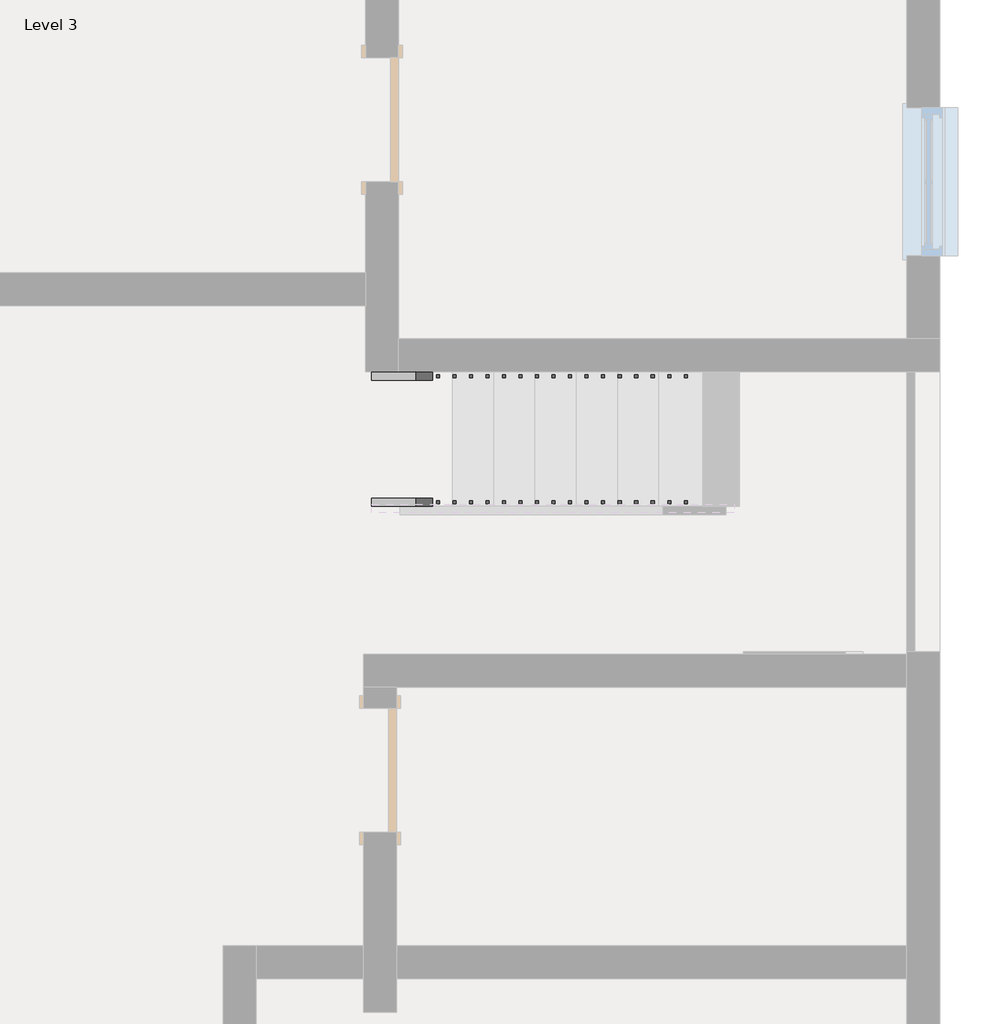
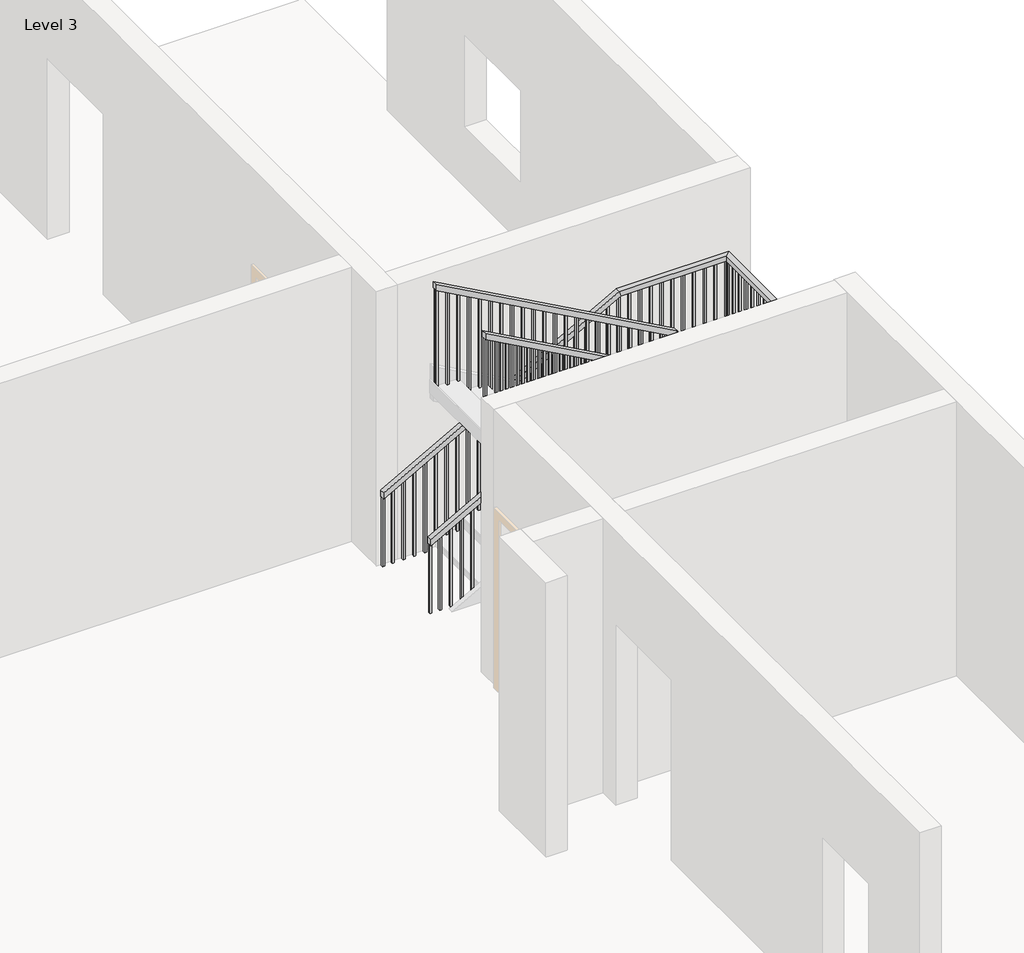
# One storey, part 3 of 4: 2 railings.
"""IFC4 building model written with IfcOpenShell, lengths in millimetres."""

from ifc_helpers import new_model, si_unit, frame, origin, place, context, project, spatial, polyline, outline, extrude, faceted_brep, element, save

model = new_model("IFC4")

# Units and contexts
model_context = context("Model", 3, world=origin())
ifc_project = project(units=[si_unit("LENGTHUNIT", "METRE", prefix="MILLI")], contexts=[model_context])

# Site, building, storey
site = spatial("IfcSite", under=ifc_project)
building = spatial("IfcBuilding", under=site)
storey = spatial("IfcBuildingStorey", under=building, Name="Level 3", Elevation=6096.0)

# Railings
placement = place(None, origin())
element("IfcRailing", 1, ObjectType="Handrail - Rectangular", at=placement, inside=storey, context=model_context, shape_type="SolidModel", body=[
    faceted_brep([(1537.1941283, 231.7547293, 7147.56), (1537.1941283, 231.7547293, 7089.4879132), (1537.1941283, 180.9547293, 7089.4879132), (1537.1941283, 180.9547293, 7147.56), (3765.8648053, 231.7547293, 8382.0), (3765.8648053, 180.9547293, 8382.0), (3765.8648053, 180.9547293, 8323.9279132), (3765.8648053, 231.7547293, 8323.9279132)], [[[0, 1, 2, 3]], [[4, 5, 6, 7]], [[1, 0, 4, 7]], [[2, 1, 7, 6]], [[3, 2, 6, 5]], [[0, 3, 5, 4]]]),
    faceted_brep([(3816.6648053, 231.7547293, 8382.0), (3816.6648053, 231.7547293, 8331.2), (3765.8648053, 231.7547293, 8331.2), (3765.8648053, 231.7547293, 8382.0), (3816.6648053, 142.8547293, 8382.0), (3765.8648053, 142.8547293, 8382.0), (3765.8648053, 92.0547293, 8331.2), (3816.6648053, 92.0547293, 8331.2)], [[[0, 1, 2, 3]], [[4, 5, 6, 7]], [[1, 0, 4, 7]], [[2, 1, 7, 6]], [[3, 2, 6, 5]], [[0, 3, 5, 4]]]),
    faceted_brep([(3816.6648053, 142.8547293, 8382.0), (3816.6648053, 92.0547293, 8331.2), (3765.8648053, 92.0547293, 8331.2), (3765.8648053, 142.8547293, 8382.0), (3816.6648053, 142.8547293, 8491.0223516), (3765.8648053, 142.8547293, 8461.0879132), (3765.8648053, 92.0547293, 8461.0879132), (3816.6648053, 92.0547293, 8491.0223516)], [[[0, 1, 2, 3]], [[4, 5, 6, 7]], [[1, 0, 4, 7]], [[2, 1, 7, 6]], [[3, 2, 6, 5]], [[0, 3, 5, 4]]]),
    faceted_brep([(3816.6648053, 92.0547293, 8491.0223516), (3765.8648053, 92.0547293, 8461.0879132), (3765.8648053, 142.8547293, 8461.0879132), (3816.6648053, 142.8547293, 8491.0223516), (1537.1941283, 92.0547293, 9753.6), (1537.1941283, 142.8547293, 9753.6), (1537.1941283, 142.8547293, 9695.5279132), (1537.1941283, 92.0547293, 9695.5279132)], [[[0, 1, 2, 3]], [[4, 5, 6, 7]], [[1, 0, 4, 7]], [[2, 1, 7, 6]], [[3, 2, 6, 5]], [[0, 3, 5, 4]]]),
    extrude(outline(polyline([(9679.7556667, 1565.5898053), (9690.3072849, 1546.5398053), (8702.04, 1546.5398053), (8702.04, 1565.5898053), (9679.7556667, 1565.5898053)])), frame((0.0, 107.9297293, 0.0), z_axis=(0.0, 1.0, 0.0), x_axis=(0.0, 0.0, 1.0)), (0.0, 0.0, 1.0), 19.05),
    extrude(outline(polyline([(9623.4803699, 1667.1898053), (9634.031988, 1648.1398053), (8702.04, 1648.1398053), (8702.04, 1667.1898053), (9623.4803699, 1667.1898053)])), frame((0.0, 107.9297293, 0.0), z_axis=(0.0, 1.0, 0.0), x_axis=(0.0, 0.0, 1.0)), (0.0, 0.0, 1.0), 19.05),
    extrude(outline(polyline([(9567.1609284, 1768.7898053), (9577.7125465, 1749.7398053), (8702.04, 1749.7398053), (8702.04, 1768.7898053), (9567.1609284, 1768.7898053)])), frame((0.0, 107.9297293, 0.0), z_axis=(0.0, 1.0, 0.0), x_axis=(0.0, 0.0, 1.0)), (0.0, 0.0, 1.0), 19.05),
    extrude(outline(polyline([(9510.9297761, 1870.3898053), (9521.4813943, 1851.3398053), (8564.88, 1851.3398053), (8564.88, 1870.3898053), (9510.9297761, 1870.3898053)])), frame((0.0, 107.9297293, 0.0), z_axis=(0.0, 1.0, 0.0), x_axis=(0.0, 0.0, 1.0)), (0.0, 0.0, 1.0), 19.05),
    extrude(outline(polyline([(9454.6544792, 1971.9898053), (9465.2060974, 1952.9398053), (8564.88, 1952.9398053), (8564.88, 1971.9898053), (9454.6544792, 1971.9898053)])), frame((0.0, 107.9297293, 0.0), z_axis=(0.0, 1.0, 0.0), x_axis=(0.0, 0.0, 1.0)), (0.0, 0.0, 1.0), 19.05),
    extrude(outline(polyline([(9398.3791823, 2073.5898053), (9408.9308005, 2054.5398053), (8427.72, 2054.5398053), (8427.72, 2073.5898053), (9398.3791823, 2073.5898053)])), frame((0.0, 107.9297293, 0.0), z_axis=(0.0, 1.0, 0.0), x_axis=(0.0, 0.0, 1.0)), (0.0, 0.0, 1.0), 19.05),
    extrude(outline(polyline([(9342.1038855, 2175.1898053), (9352.6555036, 2156.1398053), (8427.72, 2156.1398053), (8427.72, 2175.1898053), (9342.1038855, 2175.1898053)])), frame((0.0, 107.9297293, 0.0), z_axis=(0.0, 1.0, 0.0), x_axis=(0.0, 0.0, 1.0)), (0.0, 0.0, 1.0), 19.05),
    extrude(outline(polyline([(9285.8285886, 2276.7898053), (9296.3802067, 2257.7398053), (8427.72, 2257.7398053), (8427.72, 2276.7898053), (9285.8285886, 2276.7898053)])), frame((0.0, 107.9297293, 0.0), z_axis=(0.0, 1.0, 0.0), x_axis=(0.0, 0.0, 1.0)), (0.0, 0.0, 1.0), 19.05),
    extrude(outline(polyline([(9229.5532917, 2378.3898053), (9240.1049099, 2359.3398053), (8290.56, 2359.3398053), (8290.56, 2378.3898053), (9229.5532917, 2378.3898053)])), frame((0.0, 107.9297293, 0.0), z_axis=(0.0, 1.0, 0.0), x_axis=(0.0, 0.0, 1.0)), (0.0, 0.0, 1.0), 19.05),
    extrude(outline(polyline([(9173.2779948, 2479.9898053), (9183.829613, 2460.9398053), (8290.56, 2460.9398053), (8290.56, 2479.9898053), (9173.2779948, 2479.9898053)])), frame((0.0, 107.9297293, 0.0), z_axis=(0.0, 1.0, 0.0), x_axis=(0.0, 0.0, 1.0)), (0.0, 0.0, 1.0), 19.05),
    extrude(outline(polyline([(9117.0026979, 2581.5898053), (9127.5543161, 2562.5398053), (8153.4, 2562.5398053), (8153.4, 2581.5898053), (9117.0026979, 2581.5898053)])), frame((0.0, 107.9297293, 0.0), z_axis=(0.0, 1.0, 0.0), x_axis=(0.0, 0.0, 1.0)), (0.0, 0.0, 1.0), 19.05),
    extrude(outline(polyline([(9060.727401, 2683.1898053), (9071.2790192, 2664.1398053), (8153.4, 2664.1398053), (8153.4, 2683.1898053), (9060.727401, 2683.1898053)])), frame((0.0, 107.9297293, 0.0), z_axis=(0.0, 1.0, 0.0), x_axis=(0.0, 0.0, 1.0)), (0.0, 0.0, 1.0), 19.05),
    extrude(outline(polyline([(9004.4962488, 2784.7898053), (9015.0478669, 2765.7398053), (8153.4, 2765.7398053), (8153.4, 2784.7898053), (9004.4962488, 2784.7898053)])), frame((0.0, 107.9297293, 0.0), z_axis=(0.0, 1.0, 0.0), x_axis=(0.0, 0.0, 1.0)), (0.0, 0.0, 1.0), 19.05),
    extrude(outline(polyline([(8948.2209519, 2886.3898053), (8958.77257, 2867.3398053), (8016.24, 2867.3398053), (8016.24, 2886.3898053), (8948.2209519, 2886.3898053)])), frame((0.0, 107.9297293, 0.0), z_axis=(0.0, 1.0, 0.0), x_axis=(0.0, 0.0, 1.0)), (0.0, 0.0, 1.0), 19.05),
    extrude(outline(polyline([(8891.945655, 2987.9898053), (8902.4972732, 2968.9398053), (8016.24, 2968.9398053), (8016.24, 2987.9898053), (8891.945655, 2987.9898053)])), frame((0.0, 107.9297293, 0.0), z_axis=(0.0, 1.0, 0.0), x_axis=(0.0, 0.0, 1.0)), (0.0, 0.0, 1.0), 19.05),
    extrude(outline(polyline([(8835.6703581, 3089.5898053), (8846.2219763, 3070.5398053), (7879.08, 3070.5398053), (7879.08, 3089.5898053), (8835.6703581, 3089.5898053)])), frame((0.0, 107.9297293, 0.0), z_axis=(0.0, 1.0, 0.0), x_axis=(0.0, 0.0, 1.0)), (0.0, 0.0, 1.0), 19.05),
    extrude(outline(polyline([(8779.3950612, 3191.1898053), (8789.9466794, 3172.1398053), (7879.08, 3172.1398053), (7879.08, 3191.1898053), (8779.3950612, 3191.1898053)])), frame((0.0, 107.9297293, 0.0), z_axis=(0.0, 1.0, 0.0), x_axis=(0.0, 0.0, 1.0)), (0.0, 0.0, 1.0), 19.05),
    extrude(outline(polyline([(8723.1197643, 3292.7898053), (8733.6713825, 3273.7398053), (7879.08, 3273.7398053), (7879.08, 3292.7898053), (8723.1197643, 3292.7898053)])), frame((0.0, 107.9297293, 0.0), z_axis=(0.0, 1.0, 0.0), x_axis=(0.0, 0.0, 1.0)), (0.0, 0.0, 1.0), 19.05),
    extrude(outline(polyline([(8666.8444675, 3394.3898053), (8677.3960856, 3375.3398053), (7741.92, 3375.3398053), (7741.92, 3394.3898053), (8666.8444675, 3394.3898053)])), frame((0.0, 107.9297293, 0.0), z_axis=(0.0, 1.0, 0.0), x_axis=(0.0, 0.0, 1.0)), (0.0, 0.0, 1.0), 19.05),
    extrude(outline(polyline([(8610.5691706, 3495.9898053), (8621.1207888, 3476.9398053), (7741.92, 3476.9398053), (7741.92, 3495.9898053), (8610.5691706, 3495.9898053)])), frame((0.0, 107.9297293, 0.0), z_axis=(0.0, 1.0, 0.0), x_axis=(0.0, 0.0, 1.0)), (0.0, 0.0, 1.0), 19.05),
    extrude(outline(polyline([(8554.2938737, 3597.5898053), (8564.8454919, 3578.5398053), (7604.76, 3578.5398053), (7604.76, 3597.5898053), (8554.2938737, 3597.5898053)])), frame((0.0, 107.9297293, 0.0), z_axis=(0.0, 1.0, 0.0), x_axis=(0.0, 0.0, 1.0)), (0.0, 0.0, 1.0), 19.05),
    extrude(outline(polyline([(8498.0185768, 3699.1898053), (8508.570195, 3680.1398053), (7604.76, 3680.1398053), (7604.76, 3699.1898053), (8498.0185768, 3699.1898053)])), frame((0.0, 107.9297293, 0.0), z_axis=(0.0, 1.0, 0.0), x_axis=(0.0, 0.0, 1.0)), (0.0, 0.0, 1.0), 19.05),
    extrude(outline(polyline([(8332.8202537, 3781.9191283), (8322.2686355, 3762.8691283), (7467.6, 3762.8691283), (7467.6, 3781.9191283), (8332.8202537, 3781.9191283)])), frame((0.0, 196.8297293, 0.0), z_axis=(0.0, 1.0, 0.0), x_axis=(0.0, 0.0, 1.0)), (0.0, 0.0, 1.0), 19.05),
    extrude(outline(polyline([(8276.5449568, 3680.3191283), (8265.9933387, 3661.2691283), (7330.44, 3661.2691283), (7330.44, 3680.3191283), (8276.5449568, 3680.3191283)])), frame((0.0, 196.8297293, 0.0), z_axis=(0.0, 1.0, 0.0), x_axis=(0.0, 0.0, 1.0)), (0.0, 0.0, 1.0), 19.05),
    extrude(outline(polyline([(8220.2696599, 3578.7191283), (8209.7180418, 3559.6691283), (7330.44, 3559.6691283), (7330.44, 3578.7191283), (8220.2696599, 3578.7191283)])), frame((0.0, 196.8297293, 0.0), z_axis=(0.0, 1.0, 0.0), x_axis=(0.0, 0.0, 1.0)), (0.0, 0.0, 1.0), 19.05),
    extrude(outline(polyline([(8163.9943631, 3477.1191283), (8153.4427449, 3458.0691283), (7193.28, 3458.0691283), (7193.28, 3477.1191283), (8163.9943631, 3477.1191283)])), frame((0.0, 196.8297293, 0.0), z_axis=(0.0, 1.0, 0.0), x_axis=(0.0, 0.0, 1.0)), (0.0, 0.0, 1.0), 19.05),
    extrude(outline(polyline([(8107.7190662, 3375.5191283), (8097.167448, 3356.4691283), (7193.28, 3356.4691283), (7193.28, 3375.5191283), (8107.7190662, 3375.5191283)])), frame((0.0, 196.8297293, 0.0), z_axis=(0.0, 1.0, 0.0), x_axis=(0.0, 0.0, 1.0)), (0.0, 0.0, 1.0), 19.05),
    extrude(outline(polyline([(8051.4437693, 3273.9191283), (8040.8921511, 3254.8691283), (7056.12, 3254.8691283), (7056.12, 3273.9191283), (8051.4437693, 3273.9191283)])), frame((0.0, 196.8297293, 0.0), z_axis=(0.0, 1.0, 0.0), x_axis=(0.0, 0.0, 1.0)), (0.0, 0.0, 1.0), 19.05),
    extrude(outline(polyline([(7995.1684724, 3172.3191283), (7984.6168543, 3153.2691283), (7056.12, 3153.2691283), (7056.12, 3172.3191283), (7995.1684724, 3172.3191283)])), frame((0.0, 196.8297293, 0.0), z_axis=(0.0, 1.0, 0.0), x_axis=(0.0, 0.0, 1.0)), (0.0, 0.0, 1.0), 19.05),
    extrude(outline(polyline([(7938.8931755, 3070.7191283), (7928.3415574, 3051.6691283), (7056.12, 3051.6691283), (7056.12, 3070.7191283), (7938.8931755, 3070.7191283)])), frame((0.0, 196.8297293, 0.0), z_axis=(0.0, 1.0, 0.0), x_axis=(0.0, 0.0, 1.0)), (0.0, 0.0, 1.0), 19.05),
    extrude(outline(polyline([(7882.6178787, 2969.1191283), (7872.0662605, 2950.0691283), (6918.96, 2950.0691283), (6918.96, 2969.1191283), (7882.6178787, 2969.1191283)])), frame((0.0, 196.8297293, 0.0), z_axis=(0.0, 1.0, 0.0), x_axis=(0.0, 0.0, 1.0)), (0.0, 0.0, 1.0), 19.05),
    extrude(outline(polyline([(7826.3425818, 2867.5191283), (7815.7909636, 2848.4691283), (6918.96, 2848.4691283), (6918.96, 2867.5191283), (7826.3425818, 2867.5191283)])), frame((0.0, 196.8297293, 0.0), z_axis=(0.0, 1.0, 0.0), x_axis=(0.0, 0.0, 1.0)), (0.0, 0.0, 1.0), 19.05),
    extrude(outline(polyline([(7770.0672849, 2765.9191283), (7759.5156667, 2746.8691283), (6781.8, 2746.8691283), (6781.8, 2765.9191283), (7770.0672849, 2765.9191283)])), frame((0.0, 196.8297293, 0.0), z_axis=(0.0, 1.0, 0.0), x_axis=(0.0, 0.0, 1.0)), (0.0, 0.0, 1.0), 19.05),
    extrude(outline(polyline([(7713.791988, 2664.3191283), (7703.2403699, 2645.2691283), (6781.8, 2645.2691283), (6781.8, 2664.3191283), (7713.791988, 2664.3191283)])), frame((0.0, 196.8297293, 0.0), z_axis=(0.0, 1.0, 0.0), x_axis=(0.0, 0.0, 1.0)), (0.0, 0.0, 1.0), 19.05),
    extrude(outline(polyline([(7657.4725466, 2562.7191283), (7646.9209284, 2543.6691283), (6781.8, 2543.6691283), (6781.8, 2562.7191283), (7657.4725466, 2562.7191283)])), frame((0.0, 196.8297293, 0.0), z_axis=(0.0, 1.0, 0.0), x_axis=(0.0, 0.0, 1.0)), (0.0, 0.0, 1.0), 19.05),
    extrude(outline(polyline([(7601.2413943, 2461.1191283), (7590.6897761, 2442.0691283), (6644.64, 2442.0691283), (6644.64, 2461.1191283), (7601.2413943, 2461.1191283)])), frame((0.0, 196.8297293, 0.0), z_axis=(0.0, 1.0, 0.0), x_axis=(0.0, 0.0, 1.0)), (0.0, 0.0, 1.0), 19.05),
    extrude(outline(polyline([(7544.9660974, 2359.5191283), (7534.4144792, 2340.4691283), (6644.64, 2340.4691283), (6644.64, 2359.5191283), (7544.9660974, 2359.5191283)])), frame((0.0, 196.8297293, 0.0), z_axis=(0.0, 1.0, 0.0), x_axis=(0.0, 0.0, 1.0)), (0.0, 0.0, 1.0), 19.05),
    extrude(outline(polyline([(7488.6908005, 2257.9191283), (7478.1391823, 2238.8691283), (6507.48, 2238.8691283), (6507.48, 2257.9191283), (7488.6908005, 2257.9191283)])), frame((0.0, 196.8297293, 0.0), z_axis=(0.0, 1.0, 0.0), x_axis=(0.0, 0.0, 1.0)), (0.0, 0.0, 1.0), 19.05),
    extrude(outline(polyline([(7432.4155036, 2156.3191283), (7421.8638855, 2137.2691283), (6507.48, 2137.2691283), (6507.48, 2156.3191283), (7432.4155036, 2156.3191283)])), frame((0.0, 196.8297293, 0.0), z_axis=(0.0, 1.0, 0.0), x_axis=(0.0, 0.0, 1.0)), (0.0, 0.0, 1.0), 19.05),
    extrude(outline(polyline([(7376.1402067, 2054.7191283), (7365.5885886, 2035.6691283), (6507.48, 2035.6691283), (6507.48, 2054.7191283), (7376.1402067, 2054.7191283)])), frame((0.0, 196.8297293, 0.0), z_axis=(0.0, 1.0, 0.0), x_axis=(0.0, 0.0, 1.0)), (0.0, 0.0, 1.0), 19.05),
    extrude(outline(polyline([(7319.8649099, 1953.1191283), (7309.3132917, 1934.0691283), (6370.32, 1934.0691283), (6370.32, 1953.1191283), (7319.8649099, 1953.1191283)])), frame((0.0, 196.8297293, 0.0), z_axis=(0.0, 1.0, 0.0), x_axis=(0.0, 0.0, 1.0)), (0.0, 0.0, 1.0), 19.05),
    extrude(outline(polyline([(7263.589613, 1851.5191283), (7253.0379948, 1832.4691283), (6370.32, 1832.4691283), (6370.32, 1851.5191283), (7263.589613, 1851.5191283)])), frame((0.0, 196.8297293, 0.0), z_axis=(0.0, 1.0, 0.0), x_axis=(0.0, 0.0, 1.0)), (0.0, 0.0, 1.0), 19.05),
    extrude(outline(polyline([(7207.3143161, 1749.9191283), (7196.7626979, 1730.8691283), (6233.16, 1730.8691283), (6233.16, 1749.9191283), (7207.3143161, 1749.9191283)])), frame((0.0, 196.8297293, 0.0), z_axis=(0.0, 1.0, 0.0), x_axis=(0.0, 0.0, 1.0)), (0.0, 0.0, 1.0), 19.05),
    extrude(outline(polyline([(7151.0390192, 1648.3191283), (7140.487401, 1629.2691283), (6233.16, 1629.2691283), (6233.16, 1648.3191283), (7151.0390192, 1648.3191283)])), frame((0.0, 196.8297293, 0.0), z_axis=(0.0, 1.0, 0.0), x_axis=(0.0, 0.0, 1.0)), (0.0, 0.0, 1.0), 19.05),
    extrude(outline(polyline([(3781.7398053, 126.9797293), (3800.7898053, 126.9797293), (3800.7898053, 107.9297293), (3781.7398053, 107.9297293), (3781.7398053, 126.9797293)])), frame((0.0, 0.0, 7467.6), z_axis=(0.0, 0.0, 1.0), x_axis=(1.0, 0.0, 0.0)), (0.0, 0.0, 1.0), 863.6),
    extrude(outline(polyline([(8343.2725465, 3800.7898053), (8332.7209284, 3781.7398053), (7467.6, 3781.7398053), (7467.6, 3800.7898053), (8343.2725465, 3800.7898053)])), frame((0.0, 196.8297293, 0.0), z_axis=(0.0, 1.0, 0.0), x_axis=(0.0, 0.0, 1.0)), (0.0, 0.0, 1.0), 19.05),
    extrude(outline(polyline([(9684.9762951, 1556.2441283), (9695.5279132, 1537.1941283), (8702.04, 1537.1941283), (8702.04, 1556.2441283), (9684.9762951, 1556.2441283)])), frame((0.0, 107.9297293, 0.0), z_axis=(0.0, 1.0, 0.0), x_axis=(0.0, 0.0, 1.0)), (0.0, 0.0, 1.0), 19.05),
    extrude(outline(polyline([(7100.0395314, 1556.2441283), (7089.4879132, 1537.1941283), (6233.16, 1537.1941283), (6233.16, 1556.2441283), (7100.0395314, 1556.2441283)])), frame((0.0, 196.8297293, 0.0), z_axis=(0.0, 1.0, 0.0), x_axis=(0.0, 0.0, 1.0)), (0.0, 0.0, 1.0), 19.05),
])
element("IfcRailing", 2, ObjectType="Handrail - Rectangular", at=placement, inside=storey, context=model_context, shape_type="SolidModel", body=[
    faceted_brep([(1537.1941283, 1006.4547293, 7147.56), (1537.1941283, 1006.4547293, 7089.4879132), (1537.1941283, 955.6547293, 7089.4879132), (1537.1941283, 955.6547293, 7147.56), (3765.8648053, 1006.4547293, 8382.0), (3778.9939056, 1006.4547293, 8331.2), (3778.9939056, 955.6547293, 8331.2), (3765.8648053, 955.6547293, 8382.0), (4826.4941283, 1006.4547293, 8382.0), (4826.4941283, 1006.4547293, 8331.2), (4775.6941283, 955.6547293, 8331.2), (4775.6941283, 955.6547293, 8382.0), (4826.4941283, -714.2964201, 8382.0), (4826.4941283, -714.2964201, 8331.2), (4775.6941283, -663.4964201, 8331.2), (4775.6941283, -663.4964201, 8382.0), (4013.4948805, -714.2964201, 8382.0), (4000.3657803, -714.2964201, 8331.2), (4000.3657803, -663.4964201, 8331.2), (4013.4948805, -663.4964201, 8382.0), (1537.1941283, -714.2964201, 9753.6), (1537.1941283, -663.4964201, 9753.6), (1537.1941283, -663.4964201, 9695.5279132), (1537.1941283, -714.2964201, 9695.5279132)], [[[0, 1, 2, 3]], [[1, 0, 4, 5]], [[2, 1, 5, 6]], [[3, 2, 6, 7]], [[0, 3, 7, 4]], [[5, 4, 8, 9]], [[6, 5, 9, 10]], [[7, 6, 10, 11]], [[4, 7, 11, 8]], [[9, 8, 12, 13]], [[10, 9, 13, 14]], [[11, 10, 14, 15]], [[8, 11, 15, 12]], [[13, 12, 16, 17]], [[14, 13, 17, 18]], [[15, 14, 18, 19]], [[12, 15, 19, 16]], [[20, 21, 22, 23]], [[17, 16, 20, 23]], [[18, 17, 23, 22]], [[19, 18, 22, 21]], [[16, 19, 21, 20]]]),
    extrude(outline(polyline([(9693.7693102, 1540.3691283), (8702.04, 1540.3691283), (8702.04, 1559.4191283), (9683.2176921, 1559.4191283), (9693.7693102, 1540.3691283)])), frame((0.0, -698.4214201, 0.0), z_axis=(0.0, 1.0, 0.0), x_axis=(0.0, 0.0, 1.0)), (0.0, 0.0, 1.0), 19.05),
    extrude(outline(polyline([(9637.4940133, 1641.9691283), (8702.04, 1641.9691283), (8702.04, 1661.0191283), (9626.9423952, 1661.0191283), (9637.4940133, 1641.9691283)])), frame((0.0, -698.4214201, 0.0), z_axis=(0.0, 1.0, 0.0), x_axis=(0.0, 0.0, 1.0)), (0.0, 0.0, 1.0), 19.05),
    extrude(outline(polyline([(9581.2187165, 1743.5691283), (8702.04, 1743.5691283), (8702.04, 1762.6191283), (9570.6670983, 1762.6191283), (9581.2187165, 1743.5691283)])), frame((0.0, -698.4214201, 0.0), z_axis=(0.0, 1.0, 0.0), x_axis=(0.0, 0.0, 1.0)), (0.0, 0.0, 1.0), 19.05),
    extrude(outline(polyline([(9524.9434196, 1845.1691283), (8564.88, 1845.1691283), (8564.88, 1864.2191283), (9514.3918014, 1864.2191283), (9524.9434196, 1845.1691283)])), frame((0.0, -698.4214201, 0.0), z_axis=(0.0, 1.0, 0.0), x_axis=(0.0, 0.0, 1.0)), (0.0, 0.0, 1.0), 19.05),
    extrude(outline(polyline([(9468.6681227, 1946.7691283), (8564.88, 1946.7691283), (8564.88, 1965.8191283), (9458.1165045, 1965.8191283), (9468.6681227, 1946.7691283)])), frame((0.0, -698.4214201, 0.0), z_axis=(0.0, 1.0, 0.0), x_axis=(0.0, 0.0, 1.0)), (0.0, 0.0, 1.0), 19.05),
    extrude(outline(polyline([(9412.3928258, 2048.3691283), (8427.72, 2048.3691283), (8427.72, 2067.4191283), (9401.8412076, 2067.4191283), (9412.3928258, 2048.3691283)])), frame((0.0, -698.4214201, 0.0), z_axis=(0.0, 1.0, 0.0), x_axis=(0.0, 0.0, 1.0)), (0.0, 0.0, 1.0), 19.05),
    extrude(outline(polyline([(9356.1175289, 2149.9691283), (8427.72, 2149.9691283), (8427.72, 2169.0191283), (9345.5659108, 2169.0191283), (9356.1175289, 2149.9691283)])), frame((0.0, -698.4214201, 0.0), z_axis=(0.0, 1.0, 0.0), x_axis=(0.0, 0.0, 1.0)), (0.0, 0.0, 1.0), 19.05),
    extrude(outline(polyline([(9299.8422321, 2251.5691283), (8427.72, 2251.5691283), (8427.72, 2270.6191283), (9289.2906139, 2270.6191283), (9299.8422321, 2251.5691283)])), frame((0.0, -698.4214201, 0.0), z_axis=(0.0, 1.0, 0.0), x_axis=(0.0, 0.0, 1.0)), (0.0, 0.0, 1.0), 19.05),
    extrude(outline(polyline([(9243.5669352, 2353.1691283), (8290.56, 2353.1691283), (8290.56, 2372.2191283), (9233.015317, 2372.2191283), (9243.5669352, 2353.1691283)])), frame((0.0, -698.4214201, 0.0), z_axis=(0.0, 1.0, 0.0), x_axis=(0.0, 0.0, 1.0)), (0.0, 0.0, 1.0), 19.05),
    extrude(outline(polyline([(9187.2916383, 2454.7691283), (8290.56, 2454.7691283), (8290.56, 2473.8191283), (9176.7400201, 2473.8191283), (9187.2916383, 2454.7691283)])), frame((0.0, -698.4214201, 0.0), z_axis=(0.0, 1.0, 0.0), x_axis=(0.0, 0.0, 1.0)), (0.0, 0.0, 1.0), 19.05),
    extrude(outline(polyline([(9131.0163414, 2556.3691283), (8153.4, 2556.3691283), (8153.4, 2575.4191283), (9120.4647232, 2575.4191283), (9131.0163414, 2556.3691283)])), frame((0.0, -698.4214201, 0.0), z_axis=(0.0, 1.0, 0.0), x_axis=(0.0, 0.0, 1.0)), (0.0, 0.0, 1.0), 19.05),
    extrude(outline(polyline([(9074.7410445, 2657.9691283), (8153.4, 2657.9691283), (8153.4, 2677.0191283), (9064.1894264, 2677.0191283), (9074.7410445, 2657.9691283)])), frame((0.0, -698.4214201, 0.0), z_axis=(0.0, 1.0, 0.0), x_axis=(0.0, 0.0, 1.0)), (0.0, 0.0, 1.0), 19.05),
    extrude(outline(polyline([(9018.4657476, 2759.5691283), (8153.4, 2759.5691283), (8153.4, 2778.6191283), (9007.9141295, 2778.6191283), (9018.4657476, 2759.5691283)])), frame((0.0, -698.4214201, 0.0), z_axis=(0.0, 1.0, 0.0), x_axis=(0.0, 0.0, 1.0)), (0.0, 0.0, 1.0), 19.05),
    extrude(outline(polyline([(8962.3449568, 2861.1691283), (8016.24, 2861.1691283), (8016.24, 2880.2191283), (8951.7933387, 2880.2191283), (8962.3449568, 2861.1691283)])), frame((0.0, -698.4214201, 0.0), z_axis=(0.0, 1.0, 0.0), x_axis=(0.0, 0.0, 1.0)), (0.0, 0.0, 1.0), 19.05),
    extrude(outline(polyline([(8906.0696599, 2962.7691283), (8016.24, 2962.7691283), (8016.24, 2981.8191283), (8895.5180418, 2981.8191283), (8906.0696599, 2962.7691283)])), frame((0.0, -698.4214201, 0.0), z_axis=(0.0, 1.0, 0.0), x_axis=(0.0, 0.0, 1.0)), (0.0, 0.0, 1.0), 19.05),
    extrude(outline(polyline([(8849.7943631, 3064.3691283), (7879.08, 3064.3691283), (7879.08, 3083.4191283), (8839.2427449, 3083.4191283), (8849.7943631, 3064.3691283)])), frame((0.0, -698.4214201, 0.0), z_axis=(0.0, 1.0, 0.0), x_axis=(0.0, 0.0, 1.0)), (0.0, 0.0, 1.0), 19.05),
    extrude(outline(polyline([(8793.5190662, 3165.9691283), (7879.08, 3165.9691283), (7879.08, 3185.0191283), (8782.967448, 3185.0191283), (8793.5190662, 3165.9691283)])), frame((0.0, -698.4214201, 0.0), z_axis=(0.0, 1.0, 0.0), x_axis=(0.0, 0.0, 1.0)), (0.0, 0.0, 1.0), 19.05),
    extrude(outline(polyline([(8737.0892632, 3267.5691283), (7879.08, 3267.5691283), (7879.08, 3286.6191283), (8726.5376451, 3286.6191283), (8737.0892632, 3267.5691283)])), frame((0.0, -698.4214201, 0.0), z_axis=(0.0, 1.0, 0.0), x_axis=(0.0, 0.0, 1.0)), (0.0, 0.0, 1.0), 19.05),
    extrude(outline(polyline([(8680.9684724, 3369.1691283), (7741.92, 3369.1691283), (7741.92, 3388.2191283), (8670.4168543, 3388.2191283), (8680.9684724, 3369.1691283)])), frame((0.0, -698.4214201, 0.0), z_axis=(0.0, 1.0, 0.0), x_axis=(0.0, 0.0, 1.0)), (0.0, 0.0, 1.0), 19.05),
    extrude(outline(polyline([(8624.6931755, 3470.7691283), (7741.92, 3470.7691283), (7741.92, 3489.8191283), (8614.1415574, 3489.8191283), (8624.6931755, 3470.7691283)])), frame((0.0, -698.4214201, 0.0), z_axis=(0.0, 1.0, 0.0), x_axis=(0.0, 0.0, 1.0)), (0.0, 0.0, 1.0), 19.05),
    extrude(outline(polyline([(8568.4178787, 3572.3691283), (7604.76, 3572.3691283), (7604.76, 3591.4191283), (8557.8662605, 3591.4191283), (8568.4178787, 3572.3691283)])), frame((0.0, -698.4214201, 0.0), z_axis=(0.0, 1.0, 0.0), x_axis=(0.0, 0.0, 1.0)), (0.0, 0.0, 1.0), 19.05),
    extrude(outline(polyline([(8512.1425818, 3673.9691283), (7604.76, 3673.9691283), (7604.76, 3693.0191283), (8501.5909636, 3693.0191283), (8512.1425818, 3673.9691283)])), frame((0.0, -698.4214201, 0.0), z_axis=(0.0, 1.0, 0.0), x_axis=(0.0, 0.0, 1.0)), (0.0, 0.0, 1.0), 19.05),
    extrude(outline(polyline([(8455.8672849, 3775.5691283), (7467.6, 3775.5691283), (7467.6, 3794.6191283), (8445.3156667, 3794.6191283), (8455.8672849, 3775.5691283)])), frame((0.0, -698.4214201, 0.0), z_axis=(0.0, 1.0, 0.0), x_axis=(0.0, 0.0, 1.0)), (0.0, 0.0, 1.0), 19.05),
    extrude(outline(polyline([(8399.591988, 3877.1691283), (7467.6, 3877.1691283), (7467.6, 3896.2191283), (8389.0403699, 3896.2191283), (8399.591988, 3877.1691283)])), frame((0.0, -698.4214201, 0.0), z_axis=(0.0, 1.0, 0.0), x_axis=(0.0, 0.0, 1.0)), (0.0, 0.0, 1.0), 19.05),
    extrude(outline(polyline([(8343.3166911, 3978.7691283), (7467.6, 3978.7691283), (7467.6, 3997.8191283), (8332.765073, 3997.8191283), (8343.3166911, 3978.7691283)])), frame((0.0, -698.4214201, 0.0), z_axis=(0.0, 1.0, 0.0), x_axis=(0.0, 0.0, 1.0)), (0.0, 0.0, 1.0), 19.05),
    extrude(outline(polyline([(4099.4191283, -698.4214201), (4080.3691283, -698.4214201), (4080.3691283, -679.3714201), (4099.4191283, -679.3714201), (4099.4191283, -698.4214201)])), frame((0.0, 0.0, 7467.6), z_axis=(0.0, 0.0, 1.0), x_axis=(1.0, 0.0, 0.0)), (0.0, 0.0, 1.0), 863.6),
    extrude(outline(polyline([(4201.0191283, -698.4214201), (4181.9691283, -698.4214201), (4181.9691283, -679.3714201), (4201.0191283, -679.3714201), (4201.0191283, -698.4214201)])), frame((0.0, 0.0, 7467.6), z_axis=(0.0, 0.0, 1.0), x_axis=(1.0, 0.0, 0.0)), (0.0, 0.0, 1.0), 863.6),
    extrude(outline(polyline([(4302.6191283, -698.4214201), (4283.5691283, -698.4214201), (4283.5691283, -679.3714201), (4302.6191283, -679.3714201), (4302.6191283, -698.4214201)])), frame((0.0, 0.0, 7467.6), z_axis=(0.0, 0.0, 1.0), x_axis=(1.0, 0.0, 0.0)), (0.0, 0.0, 1.0), 863.6),
    extrude(outline(polyline([(4404.2191283, -698.4214201), (4385.1691283, -698.4214201), (4385.1691283, -679.3714201), (4404.2191283, -679.3714201), (4404.2191283, -698.4214201)])), frame((0.0, 0.0, 7467.6), z_axis=(0.0, 0.0, 1.0), x_axis=(1.0, 0.0, 0.0)), (0.0, 0.0, 1.0), 863.6),
    extrude(outline(polyline([(4505.8191283, -698.4214201), (4486.7691283, -698.4214201), (4486.7691283, -679.3714201), (4505.8191283, -679.3714201), (4505.8191283, -698.4214201)])), frame((0.0, 0.0, 7467.6), z_axis=(0.0, 0.0, 1.0), x_axis=(1.0, 0.0, 0.0)), (0.0, 0.0, 1.0), 863.6),
    extrude(outline(polyline([(4607.4191283, -698.4214201), (4588.3691283, -698.4214201), (4588.3691283, -679.3714201), (4607.4191283, -679.3714201), (4607.4191283, -698.4214201)])), frame((0.0, 0.0, 7467.6), z_axis=(0.0, 0.0, 1.0), x_axis=(1.0, 0.0, 0.0)), (0.0, 0.0, 1.0), 863.6),
    extrude(outline(polyline([(4709.0191283, -698.4214201), (4689.9691283, -698.4214201), (4689.9691283, -679.3714201), (4709.0191283, -679.3714201), (4709.0191283, -698.4214201)])), frame((0.0, 0.0, 7467.6), z_axis=(0.0, 0.0, 1.0), x_axis=(1.0, 0.0, 0.0)), (0.0, 0.0, 1.0), 863.6),
    extrude(outline(polyline([(4810.6191283, -635.0202707), (4810.6191283, -654.0702707), (4791.5691283, -654.0702707), (4791.5691283, -635.0202707), (4810.6191283, -635.0202707)])), frame((0.0, 0.0, 7467.6), z_axis=(0.0, 0.0, 1.0), x_axis=(1.0, 0.0, 0.0)), (0.0, 0.0, 1.0), 863.6),
    extrude(outline(polyline([(4810.6191283, -533.4202707), (4810.6191283, -552.4702707), (4791.5691283, -552.4702707), (4791.5691283, -533.4202707), (4810.6191283, -533.4202707)])), frame((0.0, 0.0, 7467.6), z_axis=(0.0, 0.0, 1.0), x_axis=(1.0, 0.0, 0.0)), (0.0, 0.0, 1.0), 863.6),
    extrude(outline(polyline([(4810.6191283, -431.8202707), (4810.6191283, -450.8702707), (4791.5691283, -450.8702707), (4791.5691283, -431.8202707), (4810.6191283, -431.8202707)])), frame((0.0, 0.0, 7467.6), z_axis=(0.0, 0.0, 1.0), x_axis=(1.0, 0.0, 0.0)), (0.0, 0.0, 1.0), 863.6),
    extrude(outline(polyline([(4810.6191283, -330.2202707), (4810.6191283, -349.2702707), (4791.5691283, -349.2702707), (4791.5691283, -330.2202707), (4810.6191283, -330.2202707)])), frame((0.0, 0.0, 7467.6), z_axis=(0.0, 0.0, 1.0), x_axis=(1.0, 0.0, 0.0)), (0.0, 0.0, 1.0), 863.6),
    extrude(outline(polyline([(4810.6191283, -228.6202707), (4810.6191283, -247.6702707), (4791.5691283, -247.6702707), (4791.5691283, -228.6202707), (4810.6191283, -228.6202707)])), frame((0.0, 0.0, 7467.6), z_axis=(0.0, 0.0, 1.0), x_axis=(1.0, 0.0, 0.0)), (0.0, 0.0, 1.0), 863.6),
    extrude(outline(polyline([(4810.6191283, -127.0202707), (4810.6191283, -146.0702707), (4791.5691283, -146.0702707), (4791.5691283, -127.0202707), (4810.6191283, -127.0202707)])), frame((0.0, 0.0, 7467.6), z_axis=(0.0, 0.0, 1.0), x_axis=(1.0, 0.0, 0.0)), (0.0, 0.0, 1.0), 863.6),
    extrude(outline(polyline([(4810.6191283, -25.4202707), (4810.6191283, -44.4702707), (4791.5691283, -44.4702707), (4791.5691283, -25.4202707), (4810.6191283, -25.4202707)])), frame((0.0, 0.0, 7467.6), z_axis=(0.0, 0.0, 1.0), x_axis=(1.0, 0.0, 0.0)), (0.0, 0.0, 1.0), 863.6),
    extrude(outline(polyline([(4810.6191283, 76.1797293), (4810.6191283, 57.1297293), (4791.5691283, 57.1297293), (4791.5691283, 76.1797293), (4810.6191283, 76.1797293)])), frame((0.0, 0.0, 7467.6), z_axis=(0.0, 0.0, 1.0), x_axis=(1.0, 0.0, 0.0)), (0.0, 0.0, 1.0), 863.6),
    extrude(outline(polyline([(4810.6191283, 177.7797293), (4810.6191283, 158.7297293), (4791.5691283, 158.7297293), (4791.5691283, 177.7797293), (4810.6191283, 177.7797293)])), frame((0.0, 0.0, 7467.6), z_axis=(0.0, 0.0, 1.0), x_axis=(1.0, 0.0, 0.0)), (0.0, 0.0, 1.0), 863.6),
    extrude(outline(polyline([(4810.6191283, 279.3797293), (4810.6191283, 260.3297293), (4791.5691283, 260.3297293), (4791.5691283, 279.3797293), (4810.6191283, 279.3797293)])), frame((0.0, 0.0, 7467.6), z_axis=(0.0, 0.0, 1.0), x_axis=(1.0, 0.0, 0.0)), (0.0, 0.0, 1.0), 863.6),
    extrude(outline(polyline([(4810.6191283, 380.9797293), (4810.6191283, 361.9297293), (4791.5691283, 361.9297293), (4791.5691283, 380.9797293), (4810.6191283, 380.9797293)])), frame((0.0, 0.0, 7467.6), z_axis=(0.0, 0.0, 1.0), x_axis=(1.0, 0.0, 0.0)), (0.0, 0.0, 1.0), 863.6),
    extrude(outline(polyline([(4810.6191283, 482.5797293), (4810.6191283, 463.5297293), (4791.5691283, 463.5297293), (4791.5691283, 482.5797293), (4810.6191283, 482.5797293)])), frame((0.0, 0.0, 7467.6), z_axis=(0.0, 0.0, 1.0), x_axis=(1.0, 0.0, 0.0)), (0.0, 0.0, 1.0), 863.6),
    extrude(outline(polyline([(4810.6191283, 584.1797293), (4810.6191283, 565.1297293), (4791.5691283, 565.1297293), (4791.5691283, 584.1797293), (4810.6191283, 584.1797293)])), frame((0.0, 0.0, 7467.6), z_axis=(0.0, 0.0, 1.0), x_axis=(1.0, 0.0, 0.0)), (0.0, 0.0, 1.0), 863.6),
    extrude(outline(polyline([(4810.6191283, 685.7797293), (4810.6191283, 666.7297293), (4791.5691283, 666.7297293), (4791.5691283, 685.7797293), (4810.6191283, 685.7797293)])), frame((0.0, 0.0, 7467.6), z_axis=(0.0, 0.0, 1.0), x_axis=(1.0, 0.0, 0.0)), (0.0, 0.0, 1.0), 863.6),
    extrude(outline(polyline([(4810.6191283, 787.3797293), (4810.6191283, 768.3297293), (4791.5691283, 768.3297293), (4791.5691283, 787.3797293), (4810.6191283, 787.3797293)])), frame((0.0, 0.0, 7467.6), z_axis=(0.0, 0.0, 1.0), x_axis=(1.0, 0.0, 0.0)), (0.0, 0.0, 1.0), 863.6),
    extrude(outline(polyline([(4810.6191283, 888.9797293), (4810.6191283, 869.9297293), (4791.5691283, 869.9297293), (4791.5691283, 888.9797293), (4810.6191283, 888.9797293)])), frame((0.0, 0.0, 7467.6), z_axis=(0.0, 0.0, 1.0), x_axis=(1.0, 0.0, 0.0)), (0.0, 0.0, 1.0), 863.6),
    extrude(outline(polyline([(4778.8691283, 990.5797293), (4797.9191283, 990.5797293), (4797.9191283, 971.5297293), (4778.8691283, 971.5297293), (4778.8691283, 990.5797293)])), frame((0.0, 0.0, 7467.6), z_axis=(0.0, 0.0, 1.0), x_axis=(1.0, 0.0, 0.0)), (0.0, 0.0, 1.0), 863.6),
    extrude(outline(polyline([(4677.2691283, 990.5797293), (4696.3191283, 990.5797293), (4696.3191283, 971.5297293), (4677.2691283, 971.5297293), (4677.2691283, 990.5797293)])), frame((0.0, 0.0, 7467.6), z_axis=(0.0, 0.0, 1.0), x_axis=(1.0, 0.0, 0.0)), (0.0, 0.0, 1.0), 863.6),
    extrude(outline(polyline([(4575.6691283, 990.5797293), (4594.7191283, 990.5797293), (4594.7191283, 971.5297293), (4575.6691283, 971.5297293), (4575.6691283, 990.5797293)])), frame((0.0, 0.0, 7467.6), z_axis=(0.0, 0.0, 1.0), x_axis=(1.0, 0.0, 0.0)), (0.0, 0.0, 1.0), 863.6),
    extrude(outline(polyline([(4474.0691283, 990.5797293), (4493.1191283, 990.5797293), (4493.1191283, 971.5297293), (4474.0691283, 971.5297293), (4474.0691283, 990.5797293)])), frame((0.0, 0.0, 7467.6), z_axis=(0.0, 0.0, 1.0), x_axis=(1.0, 0.0, 0.0)), (0.0, 0.0, 1.0), 863.6),
    extrude(outline(polyline([(4372.4691283, 990.5797293), (4391.5191283, 990.5797293), (4391.5191283, 971.5297293), (4372.4691283, 971.5297293), (4372.4691283, 990.5797293)])), frame((0.0, 0.0, 7467.6), z_axis=(0.0, 0.0, 1.0), x_axis=(1.0, 0.0, 0.0)), (0.0, 0.0, 1.0), 863.6),
    extrude(outline(polyline([(4270.8691283, 990.5797293), (4289.9191283, 990.5797293), (4289.9191283, 971.5297293), (4270.8691283, 971.5297293), (4270.8691283, 990.5797293)])), frame((0.0, 0.0, 7467.6), z_axis=(0.0, 0.0, 1.0), x_axis=(1.0, 0.0, 0.0)), (0.0, 0.0, 1.0), 863.6),
    extrude(outline(polyline([(4169.2691283, 990.5797293), (4188.3191283, 990.5797293), (4188.3191283, 971.5297293), (4169.2691283, 971.5297293), (4169.2691283, 990.5797293)])), frame((0.0, 0.0, 7467.6), z_axis=(0.0, 0.0, 1.0), x_axis=(1.0, 0.0, 0.0)), (0.0, 0.0, 1.0), 863.6),
    extrude(outline(polyline([(4067.6691283, 990.5797293), (4086.7191283, 990.5797293), (4086.7191283, 971.5297293), (4067.6691283, 971.5297293), (4067.6691283, 990.5797293)])), frame((0.0, 0.0, 7467.6), z_axis=(0.0, 0.0, 1.0), x_axis=(1.0, 0.0, 0.0)), (0.0, 0.0, 1.0), 863.6),
    extrude(outline(polyline([(3966.0691283, 990.5797293), (3985.1191283, 990.5797293), (3985.1191283, 971.5297293), (3966.0691283, 971.5297293), (3966.0691283, 990.5797293)])), frame((0.0, 0.0, 7467.6), z_axis=(0.0, 0.0, 1.0), x_axis=(1.0, 0.0, 0.0)), (0.0, 0.0, 1.0), 863.6),
    extrude(outline(polyline([(3864.4691283, 990.5797293), (3883.5191283, 990.5797293), (3883.5191283, 971.5297293), (3864.4691283, 971.5297293), (3864.4691283, 990.5797293)])), frame((0.0, 0.0, 7467.6), z_axis=(0.0, 0.0, 1.0), x_axis=(1.0, 0.0, 0.0)), (0.0, 0.0, 1.0), 863.6),
    extrude(outline(polyline([(3762.8691283, 990.5797293), (3781.9191283, 990.5797293), (3781.9191283, 971.5297293), (3762.8691283, 971.5297293), (3762.8691283, 990.5797293)])), frame((0.0, 0.0, 7467.6), z_axis=(0.0, 0.0, 1.0), x_axis=(1.0, 0.0, 0.0)), (0.0, 0.0, 1.0), 863.6),
    extrude(outline(polyline([(8265.9933387, 3661.2691283), (7330.44, 3661.2691283), (7330.44, 3680.3191283), (8276.5449568, 3680.3191283), (8265.9933387, 3661.2691283)])), frame((0.0, 971.5297293, 0.0), z_axis=(0.0, 1.0, 0.0), x_axis=(0.0, 0.0, 1.0)), (0.0, 0.0, 1.0), 19.05),
    extrude(outline(polyline([(8209.7180418, 3559.6691283), (7330.44, 3559.6691283), (7330.44, 3578.7191283), (8220.2696599, 3578.7191283), (8209.7180418, 3559.6691283)])), frame((0.0, 971.5297293, 0.0), z_axis=(0.0, 1.0, 0.0), x_axis=(0.0, 0.0, 1.0)), (0.0, 0.0, 1.0), 19.05),
    extrude(outline(polyline([(8153.4427449, 3458.0691283), (7193.28, 3458.0691283), (7193.28, 3477.1191283), (8163.9943631, 3477.1191283), (8153.4427449, 3458.0691283)])), frame((0.0, 971.5297293, 0.0), z_axis=(0.0, 1.0, 0.0), x_axis=(0.0, 0.0, 1.0)), (0.0, 0.0, 1.0), 19.05),
    extrude(outline(polyline([(8097.167448, 3356.4691283), (7193.28, 3356.4691283), (7193.28, 3375.5191283), (8107.7190662, 3375.5191283), (8097.167448, 3356.4691283)])), frame((0.0, 971.5297293, 0.0), z_axis=(0.0, 1.0, 0.0), x_axis=(0.0, 0.0, 1.0)), (0.0, 0.0, 1.0), 19.05),
    extrude(outline(polyline([(8040.8921511, 3254.8691283), (7056.12, 3254.8691283), (7056.12, 3273.9191283), (8051.4437693, 3273.9191283), (8040.8921511, 3254.8691283)])), frame((0.0, 971.5297293, 0.0), z_axis=(0.0, 1.0, 0.0), x_axis=(0.0, 0.0, 1.0)), (0.0, 0.0, 1.0), 19.05),
    extrude(outline(polyline([(7984.6168543, 3153.2691283), (7056.12, 3153.2691283), (7056.12, 3172.3191283), (7995.1684724, 3172.3191283), (7984.6168543, 3153.2691283)])), frame((0.0, 971.5297293, 0.0), z_axis=(0.0, 1.0, 0.0), x_axis=(0.0, 0.0, 1.0)), (0.0, 0.0, 1.0), 19.05),
    extrude(outline(polyline([(7928.3415574, 3051.6691283), (7056.12, 3051.6691283), (7056.12, 3070.7191283), (7938.8931755, 3070.7191283), (7928.3415574, 3051.6691283)])), frame((0.0, 971.5297293, 0.0), z_axis=(0.0, 1.0, 0.0), x_axis=(0.0, 0.0, 1.0)), (0.0, 0.0, 1.0), 19.05),
    extrude(outline(polyline([(7872.0662605, 2950.0691283), (6918.96, 2950.0691283), (6918.96, 2969.1191283), (7882.6178787, 2969.1191283), (7872.0662605, 2950.0691283)])), frame((0.0, 971.5297293, 0.0), z_axis=(0.0, 1.0, 0.0), x_axis=(0.0, 0.0, 1.0)), (0.0, 0.0, 1.0), 19.05),
    extrude(outline(polyline([(7815.7909636, 2848.4691283), (6918.96, 2848.4691283), (6918.96, 2867.5191283), (7826.3425818, 2867.5191283), (7815.7909636, 2848.4691283)])), frame((0.0, 971.5297293, 0.0), z_axis=(0.0, 1.0, 0.0), x_axis=(0.0, 0.0, 1.0)), (0.0, 0.0, 1.0), 19.05),
    extrude(outline(polyline([(7759.5156667, 2746.8691283), (6781.8, 2746.8691283), (6781.8, 2765.9191283), (7770.0672849, 2765.9191283), (7759.5156667, 2746.8691283)])), frame((0.0, 971.5297293, 0.0), z_axis=(0.0, 1.0, 0.0), x_axis=(0.0, 0.0, 1.0)), (0.0, 0.0, 1.0), 19.05),
    extrude(outline(polyline([(7703.2403699, 2645.2691283), (6781.8, 2645.2691283), (6781.8, 2664.3191283), (7713.791988, 2664.3191283), (7703.2403699, 2645.2691283)])), frame((0.0, 971.5297293, 0.0), z_axis=(0.0, 1.0, 0.0), x_axis=(0.0, 0.0, 1.0)), (0.0, 0.0, 1.0), 19.05),
    extrude(outline(polyline([(7646.965073, 2543.6691283), (6781.8, 2543.6691283), (6781.8, 2562.7191283), (7657.5166911, 2562.7191283), (7646.965073, 2543.6691283)])), frame((0.0, 971.5297293, 0.0), z_axis=(0.0, 1.0, 0.0), x_axis=(0.0, 0.0, 1.0)), (0.0, 0.0, 1.0), 19.05),
    extrude(outline(polyline([(7590.6897761, 2442.0691283), (6644.64, 2442.0691283), (6644.64, 2461.1191283), (7601.2413943, 2461.1191283), (7590.6897761, 2442.0691283)])), frame((0.0, 971.5297293, 0.0), z_axis=(0.0, 1.0, 0.0), x_axis=(0.0, 0.0, 1.0)), (0.0, 0.0, 1.0), 19.05),
    extrude(outline(polyline([(7534.4144792, 2340.4691283), (6644.64, 2340.4691283), (6644.64, 2359.5191283), (7544.9660974, 2359.5191283), (7534.4144792, 2340.4691283)])), frame((0.0, 971.5297293, 0.0), z_axis=(0.0, 1.0, 0.0), x_axis=(0.0, 0.0, 1.0)), (0.0, 0.0, 1.0), 19.05),
    extrude(outline(polyline([(7478.1391823, 2238.8691283), (6507.48, 2238.8691283), (6507.48, 2257.9191283), (7488.6908005, 2257.9191283), (7478.1391823, 2238.8691283)])), frame((0.0, 971.5297293, 0.0), z_axis=(0.0, 1.0, 0.0), x_axis=(0.0, 0.0, 1.0)), (0.0, 0.0, 1.0), 19.05),
    extrude(outline(polyline([(7421.8638855, 2137.2691283), (6507.48, 2137.2691283), (6507.48, 2156.3191283), (7432.4155036, 2156.3191283), (7421.8638855, 2137.2691283)])), frame((0.0, 971.5297293, 0.0), z_axis=(0.0, 1.0, 0.0), x_axis=(0.0, 0.0, 1.0)), (0.0, 0.0, 1.0), 19.05),
    extrude(outline(polyline([(7365.5885886, 2035.6691283), (6507.48, 2035.6691283), (6507.48, 2054.7191283), (7376.1402067, 2054.7191283), (7365.5885886, 2035.6691283)])), frame((0.0, 971.5297293, 0.0), z_axis=(0.0, 1.0, 0.0), x_axis=(0.0, 0.0, 1.0)), (0.0, 0.0, 1.0), 19.05),
    extrude(outline(polyline([(7309.3132917, 1934.0691283), (6370.32, 1934.0691283), (6370.32, 1953.1191283), (7319.8649099, 1953.1191283), (7309.3132917, 1934.0691283)])), frame((0.0, 971.5297293, 0.0), z_axis=(0.0, 1.0, 0.0), x_axis=(0.0, 0.0, 1.0)), (0.0, 0.0, 1.0), 19.05),
    extrude(outline(polyline([(7253.0379948, 1832.4691283), (6370.32, 1832.4691283), (6370.32, 1851.5191283), (7263.589613, 1851.5191283), (7253.0379948, 1832.4691283)])), frame((0.0, 971.5297293, 0.0), z_axis=(0.0, 1.0, 0.0), x_axis=(0.0, 0.0, 1.0)), (0.0, 0.0, 1.0), 19.05),
    extrude(outline(polyline([(7196.7626979, 1730.8691283), (6233.16, 1730.8691283), (6233.16, 1749.9191283), (7207.3143161, 1749.9191283), (7196.7626979, 1730.8691283)])), frame((0.0, 971.5297293, 0.0), z_axis=(0.0, 1.0, 0.0), x_axis=(0.0, 0.0, 1.0)), (0.0, 0.0, 1.0), 19.05),
    extrude(outline(polyline([(7140.487401, 1629.2691283), (6233.16, 1629.2691283), (6233.16, 1648.3191283), (7151.0390192, 1648.3191283), (7140.487401, 1629.2691283)])), frame((0.0, 971.5297293, 0.0), z_axis=(0.0, 1.0, 0.0), x_axis=(0.0, 0.0, 1.0)), (0.0, 0.0, 1.0), 19.05),
    extrude(outline(polyline([(4810.6191283, -679.3714201), (4810.6191283, -698.4214201), (4791.5691283, -698.4214201), (4791.5691283, -679.3714201), (4810.6191283, -679.3714201)])), frame((0.0, 0.0, 7467.6), z_axis=(0.0, 0.0, 1.0), x_axis=(1.0, 0.0, 0.0)), (0.0, 0.0, 1.0), 863.6),
    extrude(outline(polyline([(4791.5691283, 990.5797293), (4810.6191283, 990.5797293), (4810.6191283, 971.5297293), (4791.5691283, 971.5297293), (4791.5691283, 990.5797293)])), frame((0.0, 0.0, 7467.6), z_axis=(0.0, 0.0, 1.0), x_axis=(1.0, 0.0, 0.0)), (0.0, 0.0, 1.0), 863.6),
    extrude(outline(polyline([(9695.5279132, 1537.1941283), (8702.04, 1537.1941283), (8702.04, 1556.2441283), (9684.9762951, 1556.2441283), (9695.5279132, 1537.1941283)])), frame((0.0, -698.4214201, 0.0), z_axis=(0.0, 1.0, 0.0), x_axis=(0.0, 0.0, 1.0)), (0.0, 0.0, 1.0), 19.05),
    extrude(outline(polyline([(7089.4879132, 1537.1941283), (6233.16, 1537.1941283), (6233.16, 1556.2441283), (7100.0395314, 1556.2441283), (7089.4879132, 1537.1941283)])), frame((0.0, 971.5297293, 0.0), z_axis=(0.0, 1.0, 0.0), x_axis=(0.0, 0.0, 1.0)), (0.0, 0.0, 1.0), 19.05),
])

save(model, "model.ifc")

# Revit data of these elements
# Type "Handrail - Rectangular"
#   Assembly Code = "C2010400"
#   built-in parameter 1008612 = 0.0416667 (stored number, unit not read)
#   built-in parameter 1008611 = 0.0416667 (stored number, unit not read)
#   built-in parameter 1008609 = 0.333333 (stored number, unit not read)
#   built-in parameter 1008604 = 0.166667 (stored number, unit not read)
#   built-in parameter 1008603 = 0.166667 (stored number, unit not read)
#   Railing Height = 3' - 0"
#   built-in parameter 1008630 = 2
#   built-in parameter 1008610 = 2
#   built-in parameter 1008618 = Baluster - Square : 3/4"
# Elements 1, 2 (IfcRailing, "Handrail - Rectangular")
#   Phase Created = New Construction
